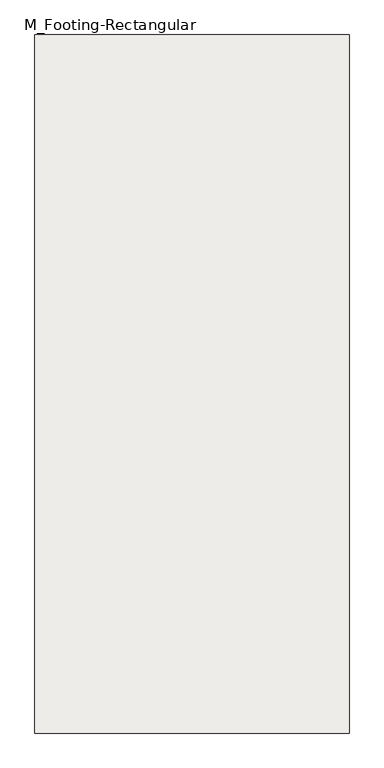
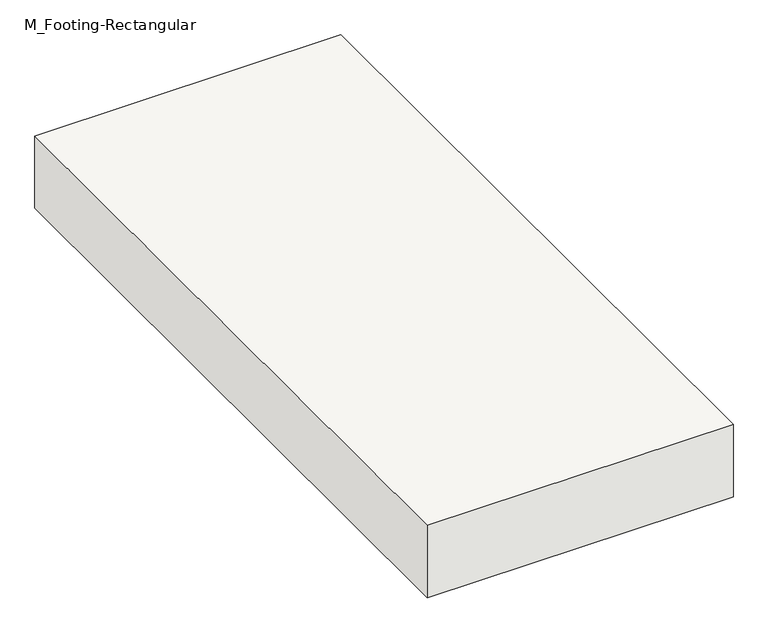
"""IFC4 building model written with IfcOpenShell, lengths in millimetres: slab geometry, M_Footing-Rectangular."""

from ifc_helpers import new_model, si_unit, frame, origin, place, context, project, spatial, polyline, outline, extrude, source, transform, mapped, element, save


def m_footing_rectangular_b51645d7(model_context):
    return source(origin(), model_context, "Body", "SweptSolid", [
        extrude(outline(polyline([(900.0, 2000.0), (900.0, -2000.0), (-900.0, -2000.0), (-900.0, 2000.0), (900.0, 2000.0)])), frame((0.0, 0.0, -450.0), z_axis=(0.0, 0.0, 1.0), x_axis=(1.0, 0.0, 0.0)), (0.0, 0.0, 1.0), 450.0),
    ])


if __name__ == "__main__":
    model = new_model("IFC4")
    model_context = context("Model", 3, world=origin())
    ifc_project = project(units=[si_unit("LENGTHUNIT", "METRE", prefix="MILLI")], contexts=[model_context])
    site = spatial("IfcSite", under=ifc_project)
    building = spatial("IfcBuilding", under=site)
    placement = place(None, origin())
    m_footing_rectangular_shape = m_footing_rectangular_b51645d7(model_context)
    element("IfcSlab", 1, ObjectType="M_Footing-Rectangular", at=placement, inside=building, context=model_context, shape_type="MappedRepresentation", body=[
        mapped(m_footing_rectangular_shape, transform((0.0, 0.0, 0.0), x_axis=(1.0, 0.0, 0.0), y_axis=(0.0, 1.0, 0.0), z_axis=(0.0, 0.0, 1.0))),
    ])
    save(model, "model.ifc")

# Revit data of these elements
# Type "M_Footing-Rectangular"
#   Width = 1800 mm
#   Length = 4000 mm
#   Foundation Thickness = 450 mm
#   Structural Material [instance default] = Concrete, Cast-in-Place gray
#   Assembly Code = ""
# Element 1 (IfcSlab, "M_Footing-Rectangular")
#   Materials on its faces: "Concrete, Cast-in-Place gray"
# Materials
#   "Concrete, Cast-in-Place gray": class "Concrete", colour RGB 192 192 192, transparency 0, Description = "Cast-in-place concrete", Cost = 0
